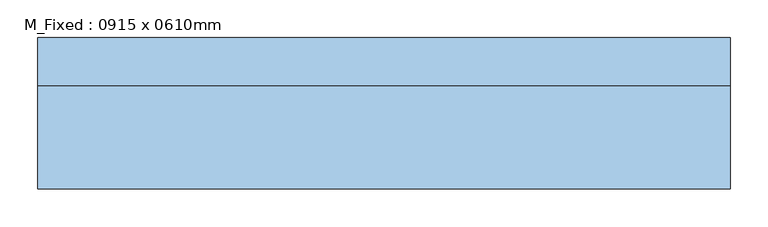
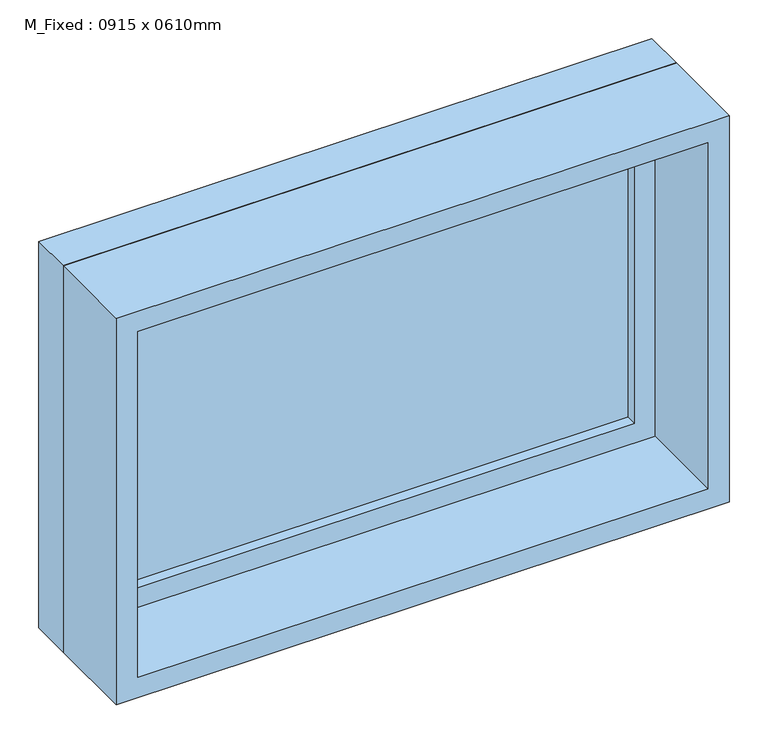
"""IFC4 building model written with IfcOpenShell, lengths in millimetres: window geometry, M_Fixed : 0915 x 0610mm."""

from ifc_helpers import new_model, si_unit, frame, origin, place, context, project, spatial, polyline, outline, extrude, source, transform, mapped, element, save


def m_fixed_0915_x_0610mm_70a843a6(model_context):
    return source(origin(), model_context, "Body", "SweptSolid", [
        extrude(outline(polyline([(-394.5, 78.0), (394.5, 78.0), (394.5, 66.0), (-394.5, 66.0), (-394.5, 78.0)])), frame((0.0, 0.0, 978.0), z_axis=(0.0, 0.0, 1.0), x_axis=(1.0, 0.0, 0.0)), (0.0, 0.0, 1.0), 484.0),
        extrude(outline(polyline([(1506.0, -438.5), (934.0, -438.5), (934.0, 438.5), (1506.0, 438.5), (1506.0, -438.5)]), holes=[polyline([(1462.0, -394.5), (1462.0, 394.5), (978.0, 394.5), (978.0, -394.5), (1462.0, -394.5)])]), frame((0.0, 50.0, 0.0), z_axis=(0.0, 1.0, 0.0), x_axis=(0.0, 0.0, 1.0)), (0.0, 0.0, 1.0), 44.0),
        extrude(outline(polyline([(1525.0, -457.5), (915.0, -457.5), (915.0, 457.5), (1525.0, 457.5), (1525.0, -457.5)]), holes=[polyline([(1506.0, -438.5), (1506.0, 438.5), (934.0, 438.5), (934.0, -438.5), (1506.0, -438.5)])]), frame((0.0, 50.0, 0.0), z_axis=(0.0, 1.0, 0.0), x_axis=(0.0, 0.0, 1.0)), (0.0, 0.0, 1.0), 63.0),
        extrude(outline(polyline([(1525.0, -457.5), (915.0, -457.5), (915.0, 457.5), (1525.0, 457.5), (1525.0, -457.5)]), holes=[polyline([(1493.0, -425.5), (1493.0, 425.5), (947.0, 425.5), (947.0, -425.5), (1493.0, -425.5)])]), frame((0.0, -87.0, 0.0), z_axis=(0.0, 1.0, 0.0), x_axis=(0.0, 0.0, 1.0)), (0.0, 0.0, 1.0), 137.0),
    ])


if __name__ == "__main__":
    model = new_model("IFC4")
    model_context = context("Model", 3, world=origin())
    ifc_project = project(units=[si_unit("LENGTHUNIT", "METRE", prefix="MILLI")], contexts=[model_context])
    site = spatial("IfcSite", under=ifc_project)
    building = spatial("IfcBuilding", under=site)
    placement = place(None, origin())
    m_fixed_0915_x_0610mm_shape = m_fixed_0915_x_0610mm_70a843a6(model_context)
    element("IfcWindow", 1, ObjectType="M_Fixed : 0915 x 0610mm", at=placement, inside=building, context=model_context, shape_type="MappedRepresentation", body=[
        mapped(m_fixed_0915_x_0610mm_shape, transform((0.0, 0.0, 0.0), x_axis=(1.0, 0.0, 0.0), y_axis=(0.0, 1.0, 0.0), z_axis=(0.0, 0.0, 1.0))),
    ])
    save(model, "model.ifc")

# Revit data of these elements
# Type "M_Fixed : 0915 x 0610mm"
#   Type Mark = "14"
#   Height = 610 mm
#   Default Sill Height = 915 mm
#   Width = 915 mm
#   Window Inset = 19 mm
#   Frame Exterior Material = Sash
#   Frame Interior Material = Sash
#   Glass Pane Material = Glass
#   Sash = Sash
#   Wall Closure = (empty or 0)
# Element 1 (IfcWindow, "M_Fixed : 0915 x 0610mm")
#   Materials on its faces: "Sash", "Glass"
# Materials
#   "Sash": class "Wood", colour RGB 136 99 55, transparency 0
#   "Glass": class "Glass", colour RGB 218 227 224, transparency 0.85, Description = "Soda Lime Glass", Cost = 0
